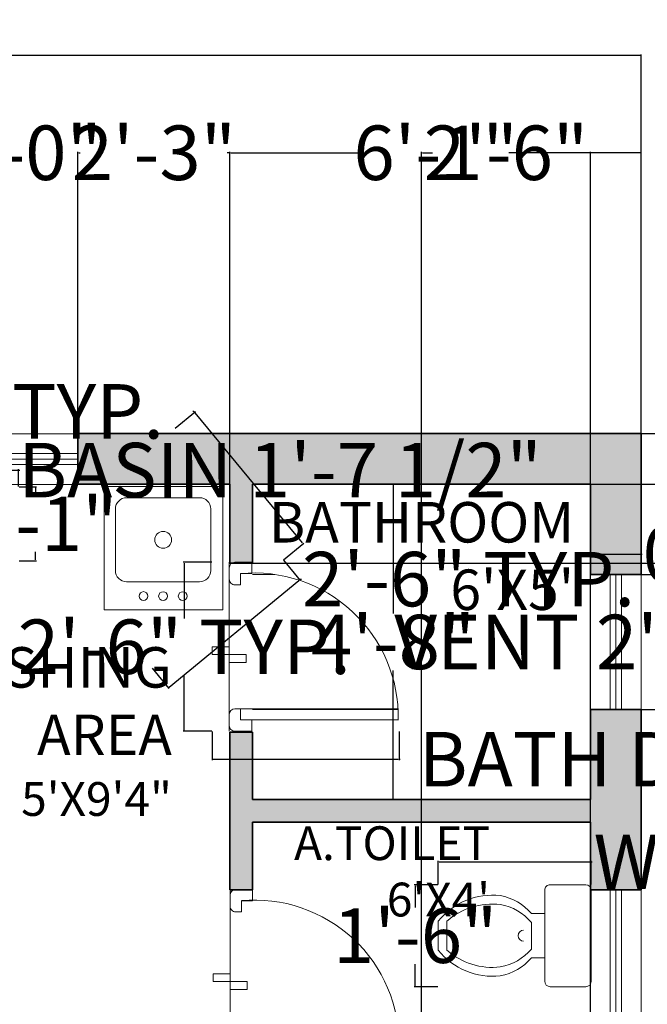
# Model space of a CAD drawing. Units: inches. Extents: x 2103 to 2702, y 2405 to 3142.
# Tile 6 of 7: x 2496 to 2607, y 2968 to 3142. Entities that reach past the tile are written whole.
import ezdxf

# ---------------------------------------------------------------- set-up
doc = ezdxf.new("R2010")
doc.units = ezdxf.units.IN
for name, color, linetype, lineweight in [('A-ANNO-DIMS', 2, 'Continuous', 18), ('A-AREA-IDEN', 7, 'Continuous', 18), ('A-FLOR-FIXT', 9, 'Continuous', 18), ('A-WALL-PATT', 8, 'Continuous', 9), ('A_FUR 1', 5, 'Continuous', 5), ('A_TEXT_SMALL', 18, 'Continuous', 5), ('doors', 4, 'Continuous', 18), ('WALL', 7, 'Continuous', 35), ('windows', 4, 'Continuous', 18)]:
    doc.layers.add(name, color=color, linetype=linetype, lineweight=lineweight)
doc.styles.get("Standard").update_dxf_attribs({"font": 'arial.ttf'})
doc.dimstyles.get("Standard").update_dxf_attribs({"dimtxt": 9.68, "dimasz": 0.18, "dimexe": 0.18, "dimexo": 0.0625, "dimgap": 0.09, "dimtad": 0, "dimtih": 1, "dimtoh": 1, "dimdec": 1, "dimzin": 0, "dimdsep": 46, "dimlunit": 3, "dimtxsty": 'Standard', "dimcen": 0.09, "dimadec": 0, "dimazin": 0, "dimtfac": 1, "dimtdec": 1, "dimtofl": 0, "dimtmove": 0, "dimatfit": 3, "dimfxl": 1, "dimtolj": 1, "dimtzin": 0, "dimarcsym": 0})

# ---------------------------------------------------------------- blocks, each defined once
blk = doc.blocks.new('ESTSET')
at = {"layer": 'A_FUR 1'}
for p, q in [((-10.44, 4.1), (-10.44, 32.1)), ((-8.44, 4.1), (-8.44, 32.1)), ((-36.44, 6.1), (-36.44, 3.1)), ((-34.44, 6.1), (-36.44, 6.1)), ((-34.44, 4.1), (-34.44, 6.1)), ((-34.44, 4.1), (-34.44, 6.1)), ((-8.44, 4.1), (-8.44, 6.1)), ((-8.44, 6.1), (-6.44, 6.1)), ((-8.44, 4.1), (-8.44, 6.1)), ((-6.44, 6.1), (-6.44, 3.1)), ((-32.44, 4.1), (-34.44, 4.1)), ((-32.44, 4.1), (-34.44, 4.1)), ((-32.44, 3.1), (-32.44, 4.1)), ((-10.44, 3.1), (-10.44, 4.1)), ((-10.44, 4.1), (-8.44, 4.1)), ((-10.44, 4.1), (-8.44, 4.1)), ((-6.44, 2.1), (-36.44, 2.1)), ((-35.44, 2.1), (-33.44, 2.1)), ((-7.44, 2.1), (-9.44, 2.1))]:
    blk.add_line(p, q, dxfattribs=at)
for points in [[(-21.44, 2.1), (-18.67, 2.1), (-18.67, 5.1), (-20.06, 5.1)], [(-20.06, 5.1), (-20.06, -0.91)], [(-21.44, 2.1), (-21.44, -0.91), (-20.06, -0.91)]]:
    blk.add_lwpolyline(points, dxfattribs=at)
for centre, radius, start, end in [((-8.91, 6.46), 25.64, 88.9606, 185.2816), ((-35.44, 3.1), 1, 180, 270), ((-33.44, 3.1), 1, 270, 0), ((-9.44, 3.1), 1, 180, 270), ((-7.44, 3.1), 1, 270, 0)]:
    blk.add_arc(centre, radius, start, end, dxfattribs=at)
blk = doc.blocks.new('ventilator')
at = {"layer": 'windows'}
for p, q in [((1922.12, 2523.05), (1898.12, 2523.05)), ((1922.12, 2522.05), (1898.12, 2522.05)), ((1922.12, 2521.05), (1898.12, 2521.05))]:
    blk.add_line(p, q, dxfattribs=at)
blk.add_lwpolyline([(1898.12, 2526.55), (1898.12, 2517.55), (1922.12, 2517.55), (1922.12, 2526.55)], close=True, dxfattribs=at)
blk = doc.blocks.new('A$C2AC94788')
for p, q in [((0.025, 0.69), (0.435, 0.69)), ((0, 0.505), (0, 0.665)), ((0.46, 0.665), (0.46, 0.505)), ((0.435, 0.48), (0.025, 0.48)), ((0.13, 0.48), (0.13, 0.42)), ((0.33, 0.42), (0.33, 0.48)), ((0.17, 0.42), (0.29, 0.42)), ((0.1641, 0.0392), (0.2959, 0.0392)), ((0.2291, 0.0392), (0.23, 0.0392)), ((0.2309, 0.0392), (0.23, 0.0392)), ((0.165, 0), (0.295, 0))]:
    blk.add_line(p, q)
for centre, radius, start, end in [((0.025, 0.665), 0.025, 90, 180), ((0.435, 0.665), 0.025, 0, 90), ((0.025, 0.505), 0.025, 180, 270), ((0.435, 0.505), 0.025, 270, 0), ((0.2874, 0.2356), 0.2425, 130.4885, 169.445), ((0.3274, 0.2356), 0.2425, 130.4885, 169.445), ((0.1326, 0.2356), 0.2425, 10.555, 49.5115), ((0.1726, 0.2356), 0.2425, 10.555, 49.5115), ((0.23, 0.385), 0.025, 180, 0), ((0.3601, 0.2448), 0.313, 173.5369, 231.4483), ((0.4001, 0.2448), 0.313, 173.5369, 221.0604), ((0.0999, 0.2448), 0.313, 308.5517, 6.4631), ((0.0599, 0.2448), 0.313, 318.9396, 6.4631)]:
    blk.add_arc(centre, radius, start, end)
blk = doc.blocks.new('reh-flat-2')
at = {"layer": 'A_TEXT_SMALL'}
for p, q in [((486053827.2, -394630231.2), (486054182.4, -394629799.8)), ((486054182.4, -394629799.8), (486054596.6, -394630140.9)), ((486054228.6, -394629903.6), (486054483.5, -394630113.5)), ((486053979.5, -394630126.3), (486054157.1, -394629910.6)), ((486054596.6, -394630140.9), (486054241.4, -394630572.3)), ((486054241.3, -394630407.7), (486053986.4, -394630197.8)), ((486054490.4, -394630185), (486054312.8, -394630400.7)), ((486054241.4, -394630572.3), (486053827.2, -394630231.2))]:
    blk.add_line(p, q, dxfattribs=at)
for centre, radius in [((486054234.9, -394630155.7), 38.1), ((486054004.1, -394630296.2), 20.1), ((486054072.7, -394630352.7), 20.1), ((486054141.4, -394630409.3), 20.1)]:
    blk.add_circle(centre, radius, dxfattribs=at)
for centre, start, end in [((486054196.3, -394629942.9), 50.5305, 140.5305), ((486054018.7, -394630158.5), 140.5305, 230.5305), ((486054451.2, -394630152.8), 320.5305, 50.5305), ((486054273.6, -394630368.4), 230.5305, 320.5305)]:
    blk.add_arc(centre, 50.8, start, end, dxfattribs=at)
blk = doc.blocks.new('*D15')
at = {"layer": 'A-ANNO-DIMS', "color": 0, "lineweight": -2, "transparency": 16777216}
for p, q in [((2246.43, 3068.91), (2246.43, 3136.18)), ((2246.61, 3136), (2418.13, 3136)), ((2606.25, 3136), (2434.73, 3136)), ((2606.43, 3068.91), (2606.43, 3136.18))]:
    blk.add_line(p, q, dxfattribs=at)
at = {"layer": 'A-ANNO-DIMS', "color": 0, "transparency": 16777216}
for points in [[(2246.61, 3136.03), (2246.61, 3135.97), (2246.43, 3136)], [(2606.25, 3136.03), (2606.25, 3135.97), (2606.43, 3136)]]:
    blk.add_solid(points, dxfattribs=at)
at = {"layer": 'Defpoints', "color": 0, "transparency": 16777216}
for p in [(2606.43, 3136), (2246.43, 3068.85), (2606.43, 3068.85)]:
    blk.add_point(p, dxfattribs=at)
at = {"layer": 'A-ANNO-DIMS', "color": 0, "transparency": 16777216, "insert": (2426.43, 3136), "char_height": 9.68, "attachment_point": 5}
blk.add_mtext("\\A1;30'", dxfattribs=at)
blk = doc.blocks.new('*D20')
at = {"layer": 'A-ANNO-DIMS', "color": 0, "lineweight": -2, "transparency": 16777216}
for p, q in [((2606.49, 3043.85), (2610.21, 3043.85)), ((2610.03, 3043.67), (2610.03, 3036.88)), ((2610.03, 3020.03), (2610.03, 3026.81)), ((2606.49, 3019.85), (2610.21, 3019.85))]:
    blk.add_line(p, q, dxfattribs=at)
at = {"layer": 'A-ANNO-DIMS', "color": 0, "transparency": 16777216}
for points in [[(2610, 3043.67), (2610.06, 3043.67), (2610.03, 3043.85)], [(2610, 3020.03), (2610.06, 3020.03), (2610.03, 3019.85)]]:
    blk.add_solid(points, dxfattribs=at)
at = {"layer": 'Defpoints', "color": 0, "transparency": 16777216}
for p in [(2606.43, 3043.85), (2606.43, 3019.85), (2610.03, 3019.85)]:
    blk.add_point(p, dxfattribs=at)
at = {"layer": 'A-ANNO-DIMS', "color": 0, "transparency": 16777216, "insert": (2610.03, 3031.85), "char_height": 9.68, "attachment_point": 5}
blk.add_mtext('\\A1;VENT 2\'-0" TYP.', dxfattribs=at)
blk = doc.blocks.new('*D21')
at = {"layer": 'A-ANNO-DIMS', "color": 0, "lineweight": -2, "transparency": 16777216}
for p, q in [((2597.43, 3043.91), (2597.43, 3047.63)), ((2597.61, 3047.45), (2606.25, 3047.45)), ((2606.43, 3043.91), (2606.43, 3047.63)), ((2606.43, 3047.45), (2606.61, 3047.45))]:
    blk.add_line(p, q, dxfattribs=at)
at = {"layer": 'A-ANNO-DIMS', "color": 0, "transparency": 16777216}
for points in [[(2597.61, 3047.48), (2597.61, 3047.42), (2597.43, 3047.45)], [(2606.25, 3047.48), (2606.25, 3047.42), (2606.43, 3047.45)]]:
    blk.add_solid(points, dxfattribs=at)
at = {"layer": 'Defpoints', "color": 0, "transparency": 16777216}
for p in [(2606.43, 3047.45), (2597.43, 3043.85), (2606.43, 3043.85)]:
    blk.add_point(p, dxfattribs=at)
at = {"layer": 'A-ANNO-DIMS', "color": 0, "transparency": 16777216, "insert": (2636.2, 3047.45), "char_height": 9.68, "attachment_point": 5}
blk.add_mtext('\\A1;0\'-9" TYP.', dxfattribs=at)
blk = doc.blocks.new('*D22')
at = {"layer": 'A-ANNO-DIMS', "color": 0, "lineweight": -2, "transparency": 16777216}
for p, q in [((2342.43, 2939.91), (2342.43, 2945.43)), ((2342.61, 2945.25), (2378.25, 2945.25)), ((2378.43, 2939.91), (2378.43, 2945.43)), ((2378.43, 2945.25), (2378.61, 2945.25))]:
    blk.add_line(p, q, dxfattribs=at)
at = {"layer": 'A-ANNO-DIMS', "color": 0, "transparency": 16777216}
for points in [[(2342.61, 2945.28), (2342.61, 2945.22), (2342.43, 2945.25)], [(2378.25, 2945.28), (2378.25, 2945.22), (2378.43, 2945.25)]]:
    blk.add_solid(points, dxfattribs=at)
at = {"layer": 'Defpoints', "color": 0, "transparency": 16777216}
for p in [(2378.43, 2945.25), (2342.43, 2939.85), (2378.43, 2939.85)]:
    blk.add_point(p, dxfattribs=at)
at = {"layer": 'A-ANNO-DIMS', "color": 0, "transparency": 16777216, "insert": (2453.03, 2945.25), "char_height": 9.68, "attachment_point": 5}
blk.add_mtext('\\A1;ROOM DOOR 3\'-0" TYP.', dxfattribs=at)
blk = doc.blocks.new('*D24')
at = {"layer": 'A-ANNO-DIMS', "color": 0, "lineweight": -2, "transparency": 16777216}
for p, q in [((2530.31, 3015.94), (2530.31, 3010.85)), ((2563.44, 3015.94), (2563.44, 3010.85)), ((2530.49, 3011.03), (2563.26, 3011.03)), ((2563.44, 3011.03), (2563.62, 3011.03))]:
    blk.add_line(p, q, dxfattribs=at)
at = {"layer": 'A-ANNO-DIMS', "color": 0, "transparency": 16777216}
for points in [[(2530.49, 3011.06), (2530.49, 3011), (2530.31, 3011.03)], [(2563.26, 3011.06), (2563.26, 3011), (2563.44, 3011.03)]]:
    blk.add_solid(points, dxfattribs=at)
at = {"layer": 'Defpoints', "color": 0, "transparency": 16777216}
for p in [(2530.31, 3016), (2563.44, 3016), (2563.44, 3011.03)]:
    blk.add_point(p, dxfattribs=at)
at = {"layer": 'A-ANNO-DIMS', "color": 0, "transparency": 16777216, "insert": (2635.08, 3011.03), "char_height": 9.68, "attachment_point": 5}
blk.add_mtext('\\A1;BATH DOOR 2\'-9" TYP.', dxfattribs=at)
blk = doc.blocks.new('*D25')
at = {"layer": 'A-ANNO-DIMS', "color": 0, "lineweight": -2, "transparency": 16777216}
for p, q in [((2530.24, 3046), (2525.16, 3046)), ((2525.34, 3045.82), (2525.34, 3036.04)), ((2525.34, 3016.18), (2525.34, 3025.97)), ((2530.24, 3016), (2525.16, 3016))]:
    blk.add_line(p, q, dxfattribs=at)
at = {"layer": 'A-ANNO-DIMS', "color": 0, "transparency": 16777216}
for points in [[(2525.31, 3045.82), (2525.37, 3045.82), (2525.34, 3046)], [(2525.31, 3016.18), (2525.37, 3016.18), (2525.34, 3016)]]:
    blk.add_solid(points, dxfattribs=at)
at = {"layer": 'Defpoints', "color": 0, "transparency": 16777216}
for p in [(2530.31, 3046), (2525.34, 3016), (2530.31, 3016)]:
    blk.add_point(p, dxfattribs=at)
at = {"layer": 'A-ANNO-DIMS', "color": 0, "transparency": 16777216, "insert": (2525.34, 3031), "char_height": 9.68, "attachment_point": 5}
blk.add_mtext('\\A1;2\'-6" TYP.', dxfattribs=at)
blk = doc.blocks.new('*D32')
at = {"layer": 'A-ANNO-DIMS', "color": 0, "lineweight": -2, "transparency": 16777216}
for p, q in [((2523.7, 3069.82), (2527.3, 3072.78)), ((2527.05, 3072.8), (2526.87, 3072.8)), ((2527.16, 3072.66), (2527.05, 3072.8)), ((2546.29, 3049.43), (2527.27, 3072.52)), ((2542.95, 3046.44), (2546.55, 3049.4))]:
    blk.add_line(p, q, dxfattribs=at)
at = {"layer": 'A-ANNO-DIMS', "color": 0, "transparency": 16777216}
for points in [[(2527.3, 3072.54), (2527.25, 3072.51), (2527.16, 3072.66)], [(2546.31, 3049.45), (2546.27, 3049.41), (2546.41, 3049.29)]]:
    blk.add_solid(points, dxfattribs=at)
at = {"layer": 'Defpoints', "color": 0, "transparency": 16777216}
for p in [(2527.16, 3072.66), (2523.65, 3069.78), (2542.9, 3046.4)]:
    blk.add_point(p, dxfattribs=at)
at = {"layer": 'A-ANNO-DIMS', "color": 0, "transparency": 16777216, "insert": (2430.03, 3072.8), "char_height": 9.68, "attachment_point": 5}
blk.add_mtext('\\A1;SINK ENVELOPE 2\'-6 1/2" TYP.', dxfattribs=at)
blk = doc.blocks.new('*D33')
at = {"layer": 'A-ANNO-DIMS', "color": 0, "lineweight": -2, "transparency": 16777216}
for p, q in [((2542.94, 3046.36), (2545.9, 3042.76)), ((2522.64, 3023.84), (2545.65, 3042.78)), ((2545.79, 3042.9), (2545.93, 3043.01)), ((2545.93, 3043.01), (2546.11, 3043.01)), ((2519.66, 3027.18), (2522.62, 3023.59))]:
    blk.add_line(p, q, dxfattribs=at)
at = {"layer": 'A-ANNO-DIMS', "color": 0, "transparency": 16777216}
for points in [[(2545.63, 3042.81), (2545.67, 3042.76), (2545.79, 3042.9)], [(2522.63, 3023.86), (2522.66, 3023.82), (2522.51, 3023.73)]]:
    blk.add_solid(points, dxfattribs=at)
at = {"layer": 'Defpoints', "color": 0, "transparency": 16777216}
for p in [(2542.9, 3046.4), (2545.79, 3042.9), (2519.62, 3027.23)]:
    blk.add_point(p, dxfattribs=at)
at = {"layer": 'A-ANNO-DIMS', "color": 0, "transparency": 16777216, "insert": (2575.78, 3043.01), "char_height": 9.68, "attachment_point": 5}
blk.add_mtext('\\A1;2\'-6" TYP.', dxfattribs=at)
blk = doc.blocks.new('*D36')
at = {"layer": 'A-ANNO-DIMS', "color": 0, "lineweight": -2, "transparency": 16777216}
for p, q in [((2570.39, 2988.81), (2570.39, 2993)), ((2570.57, 2992.82), (2597.38, 2992.82)), ((2597.56, 2988.81), (2597.56, 2993)), ((2597.56, 2992.82), (2597.74, 2992.82))]:
    blk.add_line(p, q, dxfattribs=at)
at = {"layer": 'A-ANNO-DIMS', "color": 0, "transparency": 16777216}
for points in [[(2570.57, 2992.85), (2570.57, 2992.79), (2570.39, 2992.82)], [(2597.38, 2992.85), (2597.38, 2992.79), (2597.56, 2992.82)]]:
    blk.add_solid(points, dxfattribs=at)
at = {"layer": 'Defpoints', "color": 0, "transparency": 16777216}
for p in [(2597.56, 2992.82), (2570.39, 2988.75), (2597.56, 2988.75)]:
    blk.add_point(p, dxfattribs=at)
at = {"layer": 'A-ANNO-DIMS', "color": 0, "transparency": 16777216, "insert": (2624.03, 2992.82), "char_height": 9.68, "attachment_point": 5}
blk.add_mtext('\\A1;WC 2\'-3"', dxfattribs=at)
blk = doc.blocks.new('*D37')
at = {"layer": 'A-ANNO-DIMS', "color": 0, "lineweight": -2, "transparency": 16777216}
for p, q in [((2570.33, 2988.75), (2566.13, 2988.75)), ((2566.31, 2988.57), (2566.31, 2984.72)), ((2566.31, 2970.81), (2566.31, 2974.66)), ((2570.33, 2970.63), (2566.13, 2970.63))]:
    blk.add_line(p, q, dxfattribs=at)
at = {"layer": 'A-ANNO-DIMS', "color": 0, "transparency": 16777216}
for points in [[(2566.28, 2988.57), (2566.34, 2988.57), (2566.31, 2988.75)], [(2566.28, 2970.81), (2566.34, 2970.81), (2566.31, 2970.63)]]:
    blk.add_solid(points, dxfattribs=at)
at = {"layer": 'Defpoints', "color": 0, "transparency": 16777216}
for p in [(2566.31, 2988.75), (2570.39, 2988.75), (2570.39, 2970.63)]:
    blk.add_point(p, dxfattribs=at)
at = {"layer": 'A-ANNO-DIMS', "color": 0, "transparency": 16777216, "insert": (2566.31, 2979.69), "char_height": 9.68, "attachment_point": 5}
blk.add_mtext('\\A1;1\'-6"', dxfattribs=at)
blk = doc.blocks.new('*D38')
at = {"layer": 'A-ANNO-DIMS', "color": 0, "lineweight": -2, "transparency": 16777216}
for p, q in [((2476.2, 3059.47), (2476.2, 3062.55)), ((2476.38, 3062.37), (2495.77, 3062.37)), ((2495.95, 3059.47), (2495.95, 3062.55)), ((2495.95, 3062.37), (2496.13, 3062.37))]:
    blk.add_line(p, q, dxfattribs=at)
at = {"layer": 'A-ANNO-DIMS', "color": 0, "transparency": 16777216}
for points in [[(2476.38, 3062.4), (2476.38, 3062.34), (2476.2, 3062.37)], [(2495.77, 3062.4), (2495.77, 3062.34), (2495.95, 3062.37)]]:
    blk.add_solid(points, dxfattribs=at)
at = {"layer": 'Defpoints', "color": 0, "transparency": 16777216}
for p in [(2495.95, 3062.37), (2476.2, 3059.41), (2495.95, 3059.41)]:
    blk.add_point(p, dxfattribs=at)
at = {"layer": 'A-ANNO-DIMS', "color": 0, "transparency": 16777216, "insert": (2542.32, 3062.37), "char_height": 9.68, "attachment_point": 5}
blk.add_mtext('\\A1;BASIN 1\'-7 1/2"', dxfattribs=at)
blk = doc.blocks.new('*D39')
at = {"layer": 'A-ANNO-DIMS', "color": 0, "lineweight": -2, "transparency": 16777216}
for p, q in [((2496.01, 3059.41), (2499.09, 3059.41)), ((2498.91, 3059.23), (2498.91, 3057.77)), ((2498.91, 3046.42), (2498.91, 3047.87)), ((2496.01, 3046.24), (2499.09, 3046.24))]:
    blk.add_line(p, q, dxfattribs=at)
at = {"layer": 'A-ANNO-DIMS', "color": 0, "transparency": 16777216}
for points in [[(2498.88, 3059.23), (2498.94, 3059.23), (2498.91, 3059.41)], [(2498.88, 3046.42), (2498.94, 3046.42), (2498.91, 3046.24)]]:
    blk.add_solid(points, dxfattribs=at)
at = {"layer": 'Defpoints', "color": 0, "transparency": 16777216}
for p in [(2495.95, 3059.41), (2495.95, 3046.24), (2498.91, 3046.24)]:
    blk.add_point(p, dxfattribs=at)
at = {"layer": 'A-ANNO-DIMS', "color": 0, "transparency": 16777216, "insert": (2498.91, 3052.82), "char_height": 9.68, "attachment_point": 5}
blk.add_mtext('\\A1;1\'-1"', dxfattribs=at)
blk = doc.blocks.new('*D44')
at = {"layer": 'A-ANNO-DIMS', "color": 0, "lineweight": -2, "transparency": 16777216}
for p, q in [((2471.43, 2560.91), (2471.43, 3118.9)), ((2471.61, 3118.72), (2483.25, 3118.72)), ((2483.43, 2560.91), (2483.43, 3118.9)), ((2483.43, 3118.72), (2483.61, 3118.72))]:
    blk.add_line(p, q, dxfattribs=at)
at = {"layer": 'A-ANNO-DIMS', "color": 0, "transparency": 16777216}
for points in [[(2471.61, 3118.75), (2471.61, 3118.69), (2471.43, 3118.72)], [(2483.25, 3118.75), (2483.25, 3118.69), (2483.43, 3118.72)]]:
    blk.add_solid(points, dxfattribs=at)
at = {"layer": 'Defpoints', "color": 0, "transparency": 16777216}
for p in [(2483.43, 3118.72), (2471.43, 2560.85), (2483.43, 2560.85)]:
    blk.add_point(p, dxfattribs=at)
at = {"layer": 'A-ANNO-DIMS', "color": 0, "transparency": 16777216, "insert": (2496.11, 3118.72), "char_height": 9.68, "attachment_point": 5}
blk.add_mtext('\\A1;1\'-0"', dxfattribs=at)
blk = doc.blocks.new('*D45')
at = {"layer": 'A-ANNO-DIMS', "color": 0, "lineweight": -2, "transparency": 16777216}
for p, q in [((2567.43, 2560.91), (2567.43, 3118.9)), ((2567.61, 3118.72), (2569.39, 3118.72)), ((2597.25, 3118.72), (2595.47, 3118.72)), ((2597.43, 2560.91), (2597.43, 3118.9))]:
    blk.add_line(p, q, dxfattribs=at)
at = {"layer": 'A-ANNO-DIMS', "color": 0, "transparency": 16777216}
for points in [[(2567.61, 3118.75), (2567.61, 3118.69), (2567.43, 3118.72)], [(2597.25, 3118.75), (2597.25, 3118.69), (2597.43, 3118.72)]]:
    blk.add_solid(points, dxfattribs=at)
at = {"layer": 'Defpoints', "color": 0, "transparency": 16777216}
for p in [(2597.43, 3118.72), (2567.43, 2560.85), (2597.43, 2560.85)]:
    blk.add_point(p, dxfattribs=at)
at = {"layer": 'A-ANNO-DIMS', "color": 0, "transparency": 16777216, "insert": (2582.43, 3118.72), "char_height": 9.68, "attachment_point": 5}
blk.add_mtext('\\A1;2\'-6"', dxfattribs=at)
blk = doc.blocks.new('*D57')
at = {"layer": 'A-ANNO-DIMS', "color": 0, "lineweight": -2, "transparency": 16777216}
for p, q in [((2506.43, 3059.91), (2506.43, 3118.9)), ((2506.61, 3118.72), (2506.89, 3118.72)), ((2533.25, 3118.72), (2532.97, 3118.72)), ((2533.43, 3059.91), (2533.43, 3118.9))]:
    blk.add_line(p, q, dxfattribs=at)
at = {"layer": 'A-ANNO-DIMS', "color": 0, "transparency": 16777216}
for points in [[(2506.61, 3118.75), (2506.61, 3118.69), (2506.43, 3118.72)], [(2533.25, 3118.75), (2533.25, 3118.69), (2533.43, 3118.72)]]:
    blk.add_solid(points, dxfattribs=at)
at = {"layer": 'Defpoints', "color": 0, "transparency": 16777216}
for p in [(2533.43, 3118.72), (2506.43, 3059.85), (2533.43, 3059.85)]:
    blk.add_point(p, dxfattribs=at)
at = {"layer": 'A-ANNO-DIMS', "color": 0, "transparency": 16777216, "insert": (2519.93, 3118.72), "char_height": 9.68, "attachment_point": 5}
blk.add_mtext('\\A1;2\'-3"', dxfattribs=at)
blk = doc.blocks.new('*D58')
at = {"layer": 'A-ANNO-DIMS', "color": 0, "lineweight": -2, "transparency": 16777216}
for p, q in [((2606.49, 3068.85), (2641.66, 3068.85)), ((2641.48, 3068.67), (2641.48, 3061.3)), ((2641.48, 3044.03), (2641.48, 3051.4)), ((2606.49, 3043.85), (2641.66, 3043.85))]:
    blk.add_line(p, q, dxfattribs=at)
at = {"layer": 'A-ANNO-DIMS', "color": 0, "transparency": 16777216}
for points in [[(2641.45, 3068.67), (2641.51, 3068.67), (2641.48, 3068.85)], [(2641.45, 3044.03), (2641.51, 3044.03), (2641.48, 3043.85)]]:
    blk.add_solid(points, dxfattribs=at)
at = {"layer": 'Defpoints', "color": 0, "transparency": 16777216}
for p in [(2606.43, 3068.85), (2606.43, 3043.85), (2641.48, 3043.85)]:
    blk.add_point(p, dxfattribs=at)
at = {"layer": 'A-ANNO-DIMS', "color": 0, "transparency": 16777216, "insert": (2641.48, 3056.35), "char_height": 9.68, "attachment_point": 5}
blk.add_mtext('\\A1;2\'-1"', dxfattribs=at)
blk = doc.blocks.new('*D69')
at = {"layer": 'A-ANNO-DIMS', "color": 0, "lineweight": -2, "transparency": 16777216}
for p, q in [((2537.49, 3059.85), (2641.66, 3059.85)), ((2641.48, 3059.67), (2641.48, 3057.8)), ((2641.48, 3046.03), (2641.48, 3047.9)), ((2537.49, 3045.85), (2641.66, 3045.85))]:
    blk.add_line(p, q, dxfattribs=at)
at = {"layer": 'A-ANNO-DIMS', "color": 0, "transparency": 16777216}
for points in [[(2641.45, 3059.67), (2641.51, 3059.67), (2641.48, 3059.85)], [(2641.45, 3046.03), (2641.51, 3046.03), (2641.48, 3045.85)]]:
    blk.add_solid(points, dxfattribs=at)
at = {"layer": 'Defpoints', "color": 0, "transparency": 16777216}
for p in [(2537.43, 3059.85), (2641.48, 3059.85), (2537.43, 3045.85)]:
    blk.add_point(p, dxfattribs=at)
at = {"layer": 'A-ANNO-DIMS', "color": 0, "transparency": 16777216, "insert": (2641.48, 3052.85), "char_height": 9.68, "attachment_point": 5}
blk.add_mtext('\\A1;1\'-2"', dxfattribs=at)
blk = doc.blocks.new('*D76')
at = {"layer": 'A-ANNO-DIMS', "color": 0, "lineweight": -2, "transparency": 16777216}
for p, q in [((2533.43, 3059.91), (2533.43, 3118.9)), ((2533.61, 3118.72), (2556.95, 3118.72)), ((2606.25, 3118.72), (2582.91, 3118.72)), ((2606.43, 3068.91), (2606.43, 3118.9))]:
    blk.add_line(p, q, dxfattribs=at)
at = {"layer": 'A-ANNO-DIMS', "color": 0, "transparency": 16777216}
for points in [[(2533.61, 3118.75), (2533.61, 3118.69), (2533.43, 3118.72)], [(2606.25, 3118.75), (2606.25, 3118.69), (2606.43, 3118.72)]]:
    blk.add_solid(points, dxfattribs=at)
at = {"layer": 'Defpoints', "color": 0, "transparency": 16777216}
for p in [(2606.43, 3118.72), (2606.43, 3068.85), (2533.43, 3059.85)]:
    blk.add_point(p, dxfattribs=at)
at = {"layer": 'A-ANNO-DIMS', "color": 0, "transparency": 16777216, "insert": (2569.93, 3118.72), "char_height": 9.68, "attachment_point": 5}
blk.add_mtext('\\A1;6\'-1"', dxfattribs=at)
blk = doc.blocks.new('*D77')
at = {"layer": 'A-ANNO-DIMS', "color": 0, "lineweight": -2, "transparency": 16777216}
for p, q in [((2597.37, 3059.85), (2562.2, 3059.85)), ((2562.38, 3059.67), (2562.38, 3036.88)), ((2562.38, 3004.03), (2562.38, 3026.81)), ((2597.37, 3003.85), (2562.2, 3003.85))]:
    blk.add_line(p, q, dxfattribs=at)
at = {"layer": 'A-ANNO-DIMS', "color": 0, "transparency": 16777216}
for points in [[(2562.35, 3059.67), (2562.41, 3059.67), (2562.38, 3059.85)], [(2562.35, 3004.03), (2562.41, 3004.03), (2562.38, 3003.85)]]:
    blk.add_solid(points, dxfattribs=at)
at = {"layer": 'Defpoints', "color": 0, "transparency": 16777216}
for p in [(2562.38, 3059.85), (2597.43, 3059.85), (2597.43, 3003.85)]:
    blk.add_point(p, dxfattribs=at)
at = {"layer": 'A-ANNO-DIMS', "color": 0, "transparency": 16777216, "insert": (2562.38, 3031.85), "char_height": 9.68, "attachment_point": 5}
blk.add_mtext('\\A1;4\'-8"', dxfattribs=at)

msp = doc.modelspace()

# ---------------------------------------------------------------- hatches: boundary and pattern name
at = {"layer": 'A-WALL-PATT'}
h = msp.add_hatch(color=256, dxfattribs=at)
h.dxf.hatch_style = 1
h.paths.add_polyline_path([(2255.43, 3059.85), (2289.47, 3059.85), (2289.47, 3068.85), (2289.47, 3068.85), (2246.43, 3068.85), (2246.43, 3024.23), (2255.43, 3024.23)])
h.paths.add_polyline_path([(2408.43, 3068.85), (2337.47, 3068.85), (2337.47, 3059.85), (2387.43, 3059.85), (2387.43, 3035.85), (2387.43, 2915.85), (2378.43, 2915.85), (2378.43, 2906.85), (2396.43, 2906.85), (2396.43, 3059.85), (2408.43, 3059.85), (2408.43, 3063.45)])
h.paths.add_polyline_path([(2482.43, 3068.85), (2456.43, 3068.85), (2456.43, 3059.85), (2469.43, 3059.85), (2469.43, 2999.85), (2473.43, 2999.85), (2473.43, 3003.85), (2473.43, 3059.85), (2482.43, 3059.85)])
h.paths.add_polyline_path([(2606.43, 3068.85), (2506.43, 3068.85), (2506.43, 3059.85), (2533.43, 3059.85), (2533.43, 3045.85), (2533.77, 3045.85, -0.143035), (2534.31, 3046), (2537.43, 3046), (2537.43, 3059.85), (2597.43, 3059.85), (2597.43, 3043.85), (2606.43, 3043.85)])
h = msp.add_hatch(color=256, dxfattribs=at)
h.dxf.hatch_style = 1
h.paths.add_polyline_path([(2342.43, 2911.85), (2342.43, 2915.85), (2255.43, 2915.85), (2255.43, 2976.23), (2246.43, 2976.23), (2246.43, 2840.19), (2255.43, 2840.19), (2255.43, 2854.85), (2315.43, 2854.85), (2315.43, 2845.85), (2319.43, 2845.85), (2319.43, 2858.85), (2255.43, 2858.85), (2255.43, 2906.85), (2342.43, 2906.85)])
h.paths.add_polyline_path([(2384.43, 2794.85), (2319.43, 2794.85), (2319.43, 2815.85), (2315.43, 2815.85), (2315.43, 2794.85), (2255.43, 2794.85), (2255.43, 2816.19), (2246.43, 2816.19), (2246.43, 2753.7), (2255.43, 2753.7), (2255.43, 2785.85), (2384.43, 2785.85)])
h.paths.add_polyline_path([(2606.43, 2963.85), (2597.43, 2963.85), (2597.43, 2951.85), (2537.43, 2951.85), (2537.43, 2957.85), (2533.43, 2957.85), (2533.43, 2951.85), (2469.43, 2951.85), (2444.43, 2951.85), (2444.43, 2842.85), (2449.43, 2842.85), (2453.43, 2842.85), (2453.43, 2942.85), (2597.43, 2942.85), (2597.43, 2904.89), (2606.43, 2904.89)])
h.paths.add_polyline_path([(2606.43, 3019.85), (2597.43, 3019.85), (2597.43, 3003.85), (2537.43, 3003.85), (2537.43, 3015.85), (2533.43, 3015.85), (2533.43, 2987.85), (2537.43, 2987.85), (2537.43, 2999.85), (2597.43, 2999.85), (2597.43, 2987.85), (2606.43, 2987.85)])
h.paths.add_polyline_path([(2606.43, 2856.89), (2597.43, 2856.89), (2597.43, 2774.85), (2552.43, 2774.85), (2552.43, 2765.85), (2597.43, 2765.85), (2597.43, 2749.52), (2606.43, 2749.52)])
h.paths.add_polyline_path([(2522.43, 2774.85), (2453.43, 2774.85), (2453.43, 2806.85), (2444.43, 2806.85), (2444.43, 2794.85), (2432.43, 2794.85), (2432.43, 2785.85), (2444.43, 2785.85), (2444.43, 2765.85), (2453.43, 2765.85), (2509.43, 2765.85), (2509.43, 2705.85), (2498.43, 2705.85), (2498.43, 2701.85), (2597.43, 2701.85), (2597.43, 2678.29), (2606.43, 2678.29), (2606.43, 2725.52), (2597.43, 2725.52), (2597.43, 2705.85), (2513.43, 2705.85), (2513.43, 2765.85), (2522.43, 2765.85)])
h.paths.add_polyline_path([(2255.43, 2705.7), (2246.43, 2705.7), (2246.43, 2646.55), (2255.43, 2646.55)])
h.paths.add_polyline_path([(2255.43, 2598.55), (2246.43, 2598.55), (2246.43, 2560.85), (2309.13, 2560.85), (2309.13, 2569.85), (2309.13, 2569.85), (2255.43, 2569.85)])
h.paths.add_polyline_path([(2495.43, 2569.85), (2495.43, 2569.85), (2453.43, 2569.85), (2453.43, 2701.85), (2462.43, 2701.85), (2462.43, 2705.85), (2444.43, 2705.85), (2444.43, 2569.85), (2432.43, 2569.85), (2432.43, 2564.45), (2432.43, 2564.45), (2432.43, 2560.85), (2495.43, 2560.85)])
h.paths.add_polyline_path([(2384.43, 2569.85), (2357.13, 2569.85), (2357.13, 2560.85), (2384.43, 2560.85)])
h.paths.add_polyline_path([(2606.43, 2630.29), (2597.43, 2630.29), (2597.43, 2569.85), (2543.43, 2569.85), (2543.43, 2560.85), (2597.43, 2560.85), (2597.43, 2455.85), (2450.43, 2455.85), (2450.43, 2446.85), (2606.43, 2446.85)])

# ---------------------------------------------------------------- linework, layer by layer
at = {"layer": 'doors'}
for p, q in [((2537.43, 3043.85), (2541.36, 3043.85)), ((2537.43, 3019.85), (2563.28, 3019.85)), ((2537.43, 2987.85), (2537.47, 2987.85))]:
    msp.add_line(p, q, dxfattribs=at)
at = {"layer": 'WALL'}
for p, q in [((2506.43, 3068.85), (2506.43, 3059.85)), ((2506.43, 3068.85), (2606.43, 3068.85)), ((2606.43, 3068.85), (2606.43, 3043.85)), ((2506.43, 3059.85), (2533.43, 3059.85)), ((2533.43, 3059.85), (2533.43, 3045.85)), ((2533.43, 3059.85), (2533.43, 3045.85)), ((2537.43, 3059.85), (2537.43, 3045.85)), ((2537.43, 3059.85), (2597.43, 3059.85)), ((2597.43, 3059.85), (2597.43, 3043.85)), ((2533.43, 3045.85), (2537.43, 3045.85)), ((2597.43, 3043.85), (2606.43, 3043.85)), ((2597.43, 3019.85), (2597.43, 3003.85)), ((2597.43, 3019.85), (2606.43, 3019.85)), ((2606.43, 3019.85), (2606.43, 2987.85)), ((2533.43, 3015.85), (2537.43, 3015.85)), ((2533.43, 3015.85), (2533.43, 2987.85)), ((2533.43, 3015.85), (2533.43, 3003.85)), ((2537.43, 3015.85), (2537.43, 3003.85)), ((2537.43, 3003.85), (2597.43, 3003.85)), ((2537.43, 2999.85), (2597.43, 2999.85)), ((2537.43, 2999.85), (2537.43, 2987.85)), ((2597.43, 2999.85), (2597.43, 2987.85)), ((2533.43, 2987.85), (2537.43, 2987.85)), ((2597.43, 2987.85), (2606.43, 2987.85))]:
    msp.add_line(p, q, dxfattribs=at)

# ---------------------------------------------------------------- block references
at = {"layer": 'A-FLOR-FIXT'}
for name, p, xscale, yscale, zscale, rotation in [('reh-flat-2', (-24537693.15, -166621.22), 0.0391972730482577, 0.0391972730482577, 0.0391972730482577, 39.46947596224971), ('A$C2AC94788', (2570.39, 2970.63), -39.375, 39.375, 39.375, 270)]:
    msp.add_blockref(name, p, dxfattribs=dict(at, xscale=xscale, yscale=yscale, zscale=zscale, rotation=rotation))
at = {"layer": 'doors', "rotation": 270}
for p in [(2531.22, 3009.56), (2531.37, 2951.47)]:
    msp.add_blockref('ESTSET', p, dxfattribs=at)
at = {"layer": 'windows'}
msp.add_blockref('ventilator', (584.31, 542.29), dxfattribs=at)
at = {"layer": 'windows', "rotation": 270}
for p in [(79.88, 4941.97), (79.88, 4885.97)]:
    msp.add_blockref('ventilator', p, dxfattribs=at)

# ---------------------------------------------------------------- texts
at = {"layer": 'A-AREA-IDEN', "attachment_point": 3}
for s, insert, char_height in [("BATHROOM\\P6'X5'", (2594.51, 3056.7), 7.188), ('WASHING AREA{\\H0.83478x;\\P5\'X9\'4"}', (2523.14, 3030.93), 7.1875), (" {\\H0.83478x;A.TOILET 6'X4'}", (2579.6, 2999.11), 7.1875)]:
    msp.add_mtext_dynamic_manual_height_columns(s, width=41.3807, gutter_width=12.5, heights=[0], dxfattribs=dict(at, insert=insert, char_height=char_height))

# ---------------------------------------------------------------- dimensions: what is measured, and where the dimension line sits
at = {"layer": 'A-ANNO-DIMS'}
for base, p1, p2, override, picture, middle in [((2606.43, 3136), (2246.43, 3068.85), (2606.43, 3068.85), {"dimclrd": 0, "dimclre": 0, "dimclrt": 0}, '*D15', (2426.43, 3136)), ((2483.43, 3118.72), (2471.43, 2560.85), (2483.43, 2560.85), {"dimdec": 1, "dimlfac": 1, "dimrnd": 0, "dimzin": 1, "dimdsep": 46, "dimlunit": 4, "dimfrac": 2}, '*D44', (2496.11, 3118.72)), ((2533.43, 3118.72), (2506.43, 3059.85), (2533.43, 3059.85), {"dimdec": 1, "dimlfac": 1, "dimrnd": 0, "dimzin": 1, "dimdsep": 46, "dimlunit": 4, "dimfrac": 2}, '*D57', (2519.93, 3118.72)), ((2606.43, 3118.72), (2533.43, 3059.85), (2606.43, 3068.85), {"dimdec": 1, "dimlfac": 1, "dimrnd": 0, "dimzin": 1, "dimdsep": 46, "dimlunit": 4, "dimfrac": 2}, '*D76', (2569.93, 3118.72)), ((2597.43, 3118.72), (2567.43, 2560.85), (2597.43, 2560.85), {"dimdec": 1, "dimlfac": 1, "dimrnd": 0, "dimzin": 1, "dimdsep": 46, "dimlunit": 4, "dimfrac": 2}, '*D45', (2582.43, 3118.72))]:
    dim = msp.add_linear_dim(base=base, p1=p1, p2=p2, dimstyle='Standard', override=override, dxfattribs=at)
    dim.commit()
    dim.dimension.update_dxf_attribs({"geometry": picture, "text_midpoint": middle})
for base, p1, p2, angle, text, picture, middle in [((2527.16, 3072.66), (2542.9, 3046.4), (2523.65, 3069.78), 129.4695, 'SINK ENVELOPE <> TYP.', '*D32', (2430.03, 3072.8)), ((2545.79, 3042.9), (2519.62, 3027.23), (2542.9, 3046.4), 39.4695, '<> TYP.', '*D33', (2575.78, 3043.01)), ((2610.03, 3019.85), (2606.43, 3043.85), (2606.43, 3019.85), 270, 'VENT <> TYP.', '*D20', (2610.03, 3031.85)), ((2525.34, 3016), (2530.31, 3046), (2530.31, 3016), 270, '<> TYP.', '*D25', (2525.34, 3031)), ((2378.43, 2945.25), (2342.43, 2939.85), (2378.43, 2939.85), 360, 'ROOM DOOR <> TYP.', '*D22', (2453.03, 2945.25))]:
    dim = msp.add_linear_dim(base=base, p1=p1, p2=p2, angle=angle, text=text, dimstyle='Standard', override={"dimdec": 1, "dimlfac": 1, "dimrnd": 0, "dimzin": 1, "dimdsep": 46, "dimlunit": 4, "dimfrac": 2}, dxfattribs=at)
    dim.commit()
    dim.dimension.update_dxf_attribs({"geometry": picture, "text_midpoint": middle})
for base, p1, p2, text, picture, middle in [((2495.9471, 3062.3675), (2476.2014, 3059.4057), (2495.9471, 3059.4057), 'BASIN <>', '*D38', (2542.3159, 3062.3675)), ((2606.43, 3047.45), (2597.43, 3043.85), (2606.43, 3043.85), '<> TYP.', '*D21', (2636.2, 3047.45)), ((2563.44, 3011.03), (2530.31, 3016), (2563.44, 3016), 'BATH DOOR <> TYP.', '*D24', (2635.08, 3011.03)), ((2597.56, 2992.82), (2570.39, 2988.75), (2597.56, 2988.75), 'WC <>', '*D36', (2624.03, 2992.82))]:
    dim = msp.add_linear_dim(base=base, p1=p1, p2=p2, text=text, dimstyle='Standard', override={"dimdec": 1, "dimlfac": 1, "dimrnd": 0, "dimzin": 1, "dimdsep": 46, "dimlunit": 4, "dimfrac": 2}, dxfattribs=at)
    dim.commit()
    dim.dimension.update_dxf_attribs({"geometry": picture, "text_midpoint": middle})
for base, p1, p2, angle, picture, middle in [((2641.48, 3043.85), (2606.43, 3068.85), (2606.43, 3043.85), 90, '*D58', (2641.48, 3056.35)), ((2498.91, 3046.24), (2495.95, 3059.41), (2495.95, 3046.24), 270, '*D39', (2498.91, 3052.82)), ((2641.48, 3059.85), (2537.43, 3045.85), (2537.43, 3059.85), 90, '*D69', (2641.48, 3052.85)), ((2562.38, 3059.85), (2597.43, 3003.85), (2597.43, 3059.85), 90, '*D77', (2562.38, 3031.85)), ((2566.31, 2988.75), (2570.39, 2970.63), (2570.39, 2988.75), 90, '*D37', (2566.31, 2979.69))]:
    dim = msp.add_linear_dim(base=base, p1=p1, p2=p2, angle=angle, dimstyle='Standard', override={"dimdec": 1, "dimlfac": 1, "dimrnd": 0, "dimzin": 1, "dimdsep": 46, "dimlunit": 4, "dimfrac": 2}, dxfattribs=at)
    dim.commit()
    dim.dimension.update_dxf_attribs({"geometry": picture, "text_midpoint": middle})

doc.saveas('drawing.dxf')
